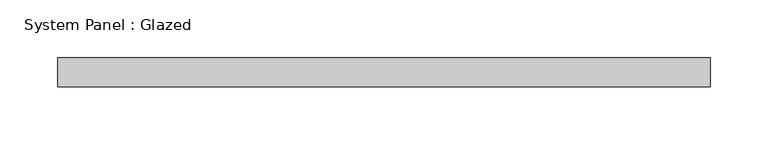
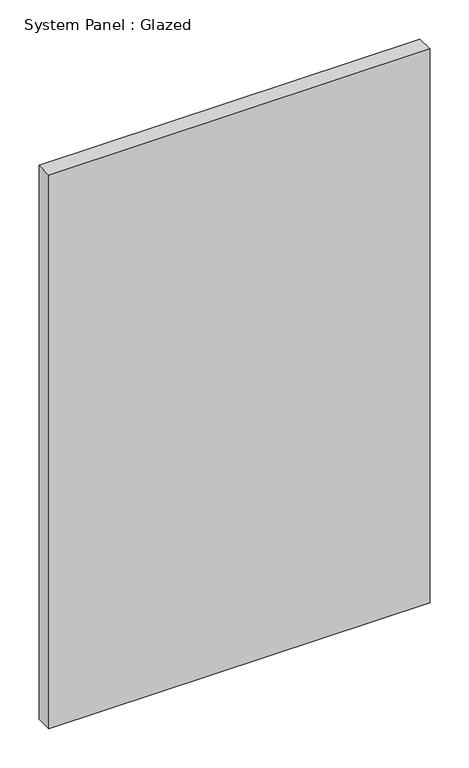
"""IFC4 building model written with IfcOpenShell, lengths in millimetres: plate geometry, System Panel : Glazed."""

from ifc_helpers import new_model, si_unit, origin, origin_with_axes, place, context, project, spatial, polyline, outline, extrude, source, transform, mapped, element, save


def system_panel_glazed_8bec2438(model_context):
    return source(origin(), model_context, "Body", "SweptSolid", [
        extrude(outline(polyline([(281.5166667, 24.5), (-281.5166667, 24.5), (-281.5166667, 49.5), (281.5166667, 49.5), (281.5166667, 24.5)])), origin_with_axes(), (0.0, 0.0, 1.0), 864.4),
    ])


if __name__ == "__main__":
    model = new_model("IFC4")
    model_context = context("Model", 3, world=origin())
    ifc_project = project(units=[si_unit("LENGTHUNIT", "METRE", prefix="MILLI")], contexts=[model_context])
    site = spatial("IfcSite", under=ifc_project)
    building = spatial("IfcBuilding", under=site)
    placement = place(None, origin())
    system_panel_glazed_shape = system_panel_glazed_8bec2438(model_context)
    element("IfcPlate", 1, ObjectType="System Panel : Glazed", at=placement, inside=building, context=model_context, shape_type="MappedRepresentation", body=[
        mapped(system_panel_glazed_shape, transform((0.0, 0.0, 0.0), x_axis=(1.0, 0.0, 0.0), y_axis=(0.0, 1.0, 0.0), z_axis=(0.0, 0.0, 1.0))),
    ])
    save(model, "model.ifc")

# Revit data of these elements
# Type "System Panel : Glazed"
#   Keynote = "H11"
#   Construction Type Id = "GSP4R"
#   Analytic Construction = "1/8 in Pilkington single glazing"
#   Visual Light Transmittance = 0.9
#   Solar Heat Gain Coefficient = 0.86
#   Heat Transfer Coefficient (U) = 6.7069 W/(m²·K)
#   Define Thermal Properties by = 1
# Element 1 (IfcPlate, "System Panel : Glazed")
#   Materials on its faces: "Glass"
# Materials
#   "Glass": class "Glass", colour RGB 0 128 192, transparency 0.9, Description = "Soda Lime Glass", Cost = 0
